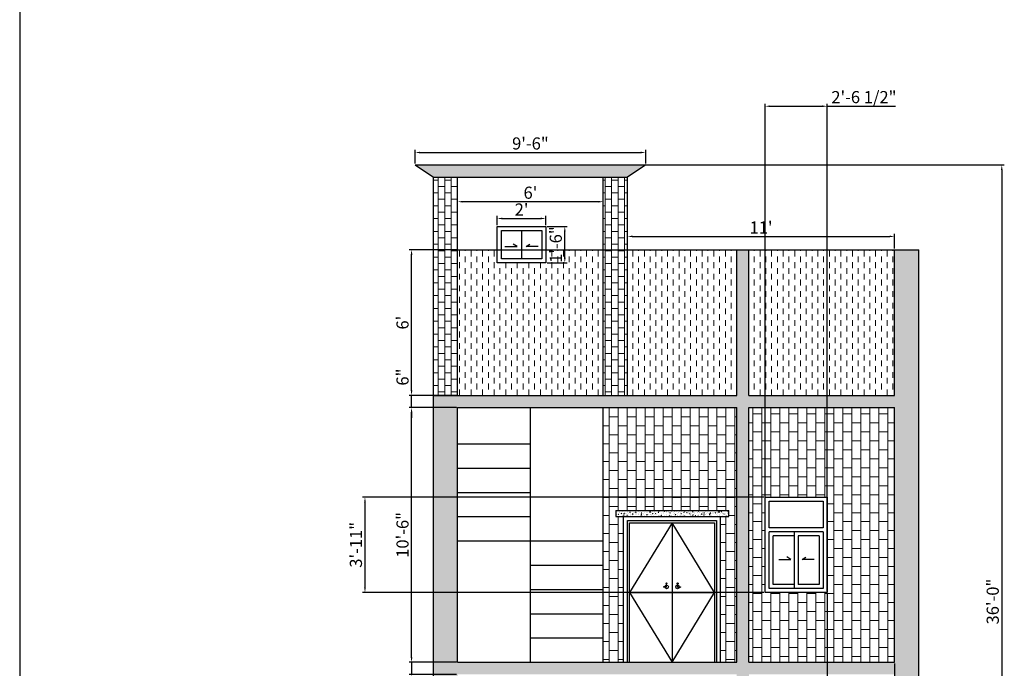
# Model space of a CAD drawing. Units: millimetres. Extents: x 20768 to 23556, y 50760 to 52704.
# Tile 5 of 36: x 20768 to 21255, y 51283 to 51604. Entities that reach past the tile are written whole.
import ezdxf

# ---------------------------------------------------------------- set-up
doc = ezdxf.new("R2010")
doc.units = ezdxf.units.MM
for name, color, linetype, lineweight in [('A-ANNO-DIMS', 2, 'Continuous', 18), ('A-ELEV', 7, 'Continuous', 25), ('A-ELEV-PATT', 8, 'Continuous', 13), ('S-ANNO-DIMS', 2, 'Continuous', 18)]:
    doc.layers.add(name, color=color, linetype=linetype, lineweight=lineweight)
doc.styles.get("Standard").update_dxf_attribs({"font": 'arial.ttf'})
doc.dimstyles.new('ISO-25', dxfattribs={"dimtxt": 6, "dimasz": 2.5, "dimexe": 1.25, "dimexo": 0.625, "dimtad": 1, "dimdec": 0, "dimlunit": 3, "dimtxsty": 'Standard', "dimcen": 2.5, "dimadec": 0, "dimazin": 0, "dimtfac": 1, "dimtdec": 0, "dimtmove": 0, "dimatfit": 3, "dimfxl": 1, "dimarcsym": 0})
pattern_1 = [(90, (105.777, 340.6355), (-3.175, 2e-16), []), (180, (105.777, 340.6355), (-8e-16, -6.35), [3.175, -3.175]), (180, (105.777, 343.8105), (-8e-16, -6.35), [-3.175, 3.175])]
pattern_2 = [(90, (105.777, 340.6355), (-2.8575, 2.8575), [2.8575, -2.8575])]
pattern_3 = [(140, (105.777, 340.6355), (0.23908628, 2.732770035), [0.28575, -3.14325]), (85, (105.777, 340.6355), (-2.86585268, -0.52865132), [0.2286, -2.51460876]), (190.4514447, (105.797, 340.8633), (-2.62676628, 2.20411871), [0.24285013, -2.67135367]), (136.1842, (105.015, 340.6355), (0.63063492, 4.06618561), [0.428625, -4.714875]), (186.635558, (105.0677, 340.9744), (-3.71139187, 3.561062), [0.36427535, -4.00703412]), (81.184151, (105.015, 340.6355), (-3.71139187, 3.561062), [0.3428995, -3.77189598]), (111, (105.2056, 341.0165), (1.53397797, 2.27421587), [0.28575, -3.14325]), (56, (105.2056, 341.0165), (-2.76281949, 0.92703043), [0.2286, -2.5146]), (161.451445, (105.3334, 341.206), (-1.22884153, 3.20124629), [0.24285013, -2.67134906]), (127.5, (105.7771, 340.6355), (-1.268325583, 0.046329049), [0, -2.48412, 0, -2.5527, 0, -2.524125]), (97.5, (105.7771, 340.6355), (-1.502708622, 1.002294938), [0, -1.45542, 0, -2.42697, 0, -0.962025]), (57.5, (105.7771, 339.7859), (0.08593116, 2.033858928), [0, -0.9525, 0, -2.9718, 0, -3.94335]), (47.5, (105.7771, 339.4049), (-0.381397365, 2.22193772), [0, -1.23825, 0, -1.97358, 0, -2.80035])]

# ---------------------------------------------------------------- blocks, each defined once
blk = doc.blocks.new('*D115')
at = {"layer": 'A-ANNO-DIMS', "color": 0, "lineweight": -2, "transparency": 16777216}
for p, q in [((20961.86, 51288.9), (20961.86, 51291.4)), ((20984.01, 51286.4), (20960.61, 51286.4)), ((20961.86, 51286.4), (20961.86, 51280.4)), ((20984.01, 51280.4), (20960.61, 51280.4)), ((20961.86, 51277.9), (20961.86, 51267.22))]:
    blk.add_line(p, q, dxfattribs=at)
at = {"layer": 'A-ANNO-DIMS', "color": 0, "transparency": 16777216}
for points in [[(20961.44, 51288.9), (20962.28, 51288.9), (20961.86, 51286.4)], [(20961.44, 51277.9), (20962.28, 51277.9), (20961.86, 51280.4)]]:
    blk.add_solid(points, dxfattribs=at)
at = {"layer": 'Defpoints', "color": 0, "transparency": 16777216}
for p in [(20984.63, 51286.4), (20961.86, 51280.4), (20984.63, 51280.4)]:
    blk.add_point(p, dxfattribs=at)
at = {"layer": 'A-ANNO-DIMS', "color": 0, "transparency": 16777216, "insert": (20958.17, 51271.31), "char_height": 6, "attachment_point": 5, "rotation": 90}
blk.add_mtext('6"', dxfattribs=at)
blk = doc.blocks.new('*D116')
at = {"layer": 'A-ANNO-DIMS', "color": 0, "lineweight": -2, "transparency": 16777216}
for p, q in [((20984.01, 51412.3), (20960.61, 51412.3)), ((20961.86, 51288.9), (20961.86, 51409.8)), ((20984.01, 51286.4), (20960.61, 51286.4))]:
    blk.add_line(p, q, dxfattribs=at)
at = {"layer": 'A-ANNO-DIMS', "color": 0, "transparency": 16777216}
for points in [[(20961.44, 51409.8), (20962.28, 51409.8), (20961.86, 51412.3)], [(20961.44, 51288.9), (20962.28, 51288.9), (20961.86, 51286.4)]]:
    blk.add_solid(points, dxfattribs=at)
at = {"layer": 'Defpoints', "color": 0, "transparency": 16777216}
for p in [(20961.86, 51412.3), (20984.63, 51412.3), (20984.63, 51286.4)]:
    blk.add_point(p, dxfattribs=at)
at = {"layer": 'A-ANNO-DIMS', "color": 0, "transparency": 16777216, "insert": (20958.17, 51349.35), "char_height": 6, "attachment_point": 5, "rotation": 90}
blk.add_mtext('10\'-6"', dxfattribs=at)
blk = doc.blocks.new('*D117')
at = {"layer": 'A-ANNO-DIMS', "color": 0, "lineweight": -2, "transparency": 16777216}
for p, q in [((20961.86, 51420.8), (20961.86, 51431.48)), ((20984.01, 51418.3), (20960.61, 51418.3)), ((20961.86, 51412.3), (20961.86, 51418.3)), ((20984.01, 51412.3), (20960.61, 51412.3)), ((20961.86, 51409.8), (20961.86, 51407.3))]:
    blk.add_line(p, q, dxfattribs=at)
at = {"layer": 'A-ANNO-DIMS', "color": 0, "transparency": 16777216}
for points in [[(20961.44, 51420.8), (20962.28, 51420.8), (20961.86, 51418.3)], [(20961.44, 51409.8), (20962.28, 51409.8), (20961.86, 51412.3)]]:
    blk.add_solid(points, dxfattribs=at)
at = {"layer": 'Defpoints', "color": 0, "transparency": 16777216}
for p in [(20961.86, 51418.3), (20984.63, 51418.3), (20984.63, 51412.3)]:
    blk.add_point(p, dxfattribs=at)
at = {"layer": 'A-ANNO-DIMS', "color": 0, "transparency": 16777216, "insert": (20958.17, 51427.39), "char_height": 6, "attachment_point": 5, "rotation": 90}
blk.add_mtext('6"', dxfattribs=at)
blk = doc.blocks.new('*D118')
at = {"layer": 'A-ANNO-DIMS', "color": 0, "lineweight": -2, "transparency": 16777216}
for p, q in [((21004.25, 51502.51), (21004.25, 51507.06)), ((21028.25, 51502.51), (21028.25, 51507.06)), ((21006.75, 51505.81), (21025.75, 51505.81))]:
    blk.add_line(p, q, dxfattribs=at)
at = {"layer": 'A-ANNO-DIMS', "color": 0, "transparency": 16777216}
for points in [[(21006.75, 51506.22), (21006.75, 51505.39), (21004.25, 51505.81)], [(21025.75, 51506.22), (21025.75, 51505.39), (21028.25, 51505.81)]]:
    blk.add_solid(points, dxfattribs=at)
at = {"layer": 'Defpoints', "color": 0, "transparency": 16777216}
for p in [(21028.25, 51505.81), (21004.25, 51501.88), (21028.25, 51501.88)]:
    blk.add_point(p, dxfattribs=at)
at = {"layer": 'A-ANNO-DIMS', "color": 0, "transparency": 16777216, "insert": (21016.25, 51509.45), "char_height": 6, "attachment_point": 5}
blk.add_mtext("2'", dxfattribs=at)
blk = doc.blocks.new('*D119')
at = {"layer": 'A-ANNO-DIMS', "color": 0, "lineweight": -2, "transparency": 16777216}
for p, q in [((21028.87, 51501.88), (21038.86, 51501.88)), ((21037.61, 51486.38), (21037.61, 51499.38)), ((21028.87, 51483.88), (21038.86, 51483.88))]:
    blk.add_line(p, q, dxfattribs=at)
at = {"layer": 'A-ANNO-DIMS', "color": 0, "transparency": 16777216}
for points in [[(21037.2, 51499.38), (21038.03, 51499.38), (21037.61, 51501.88)], [(21037.2, 51486.38), (21038.03, 51486.38), (21037.61, 51483.88)]]:
    blk.add_solid(points, dxfattribs=at)
at = {"layer": 'Defpoints', "color": 0, "transparency": 16777216}
for p in [(21028.25, 51501.88), (21037.61, 51501.88), (21028.25, 51483.88)]:
    blk.add_point(p, dxfattribs=at)
at = {"layer": 'A-ANNO-DIMS', "color": 0, "transparency": 16777216, "insert": (21033.93, 51492.88), "char_height": 6, "attachment_point": 5, "rotation": 90}
blk.add_mtext('1\'-6"', dxfattribs=at)
blk = doc.blocks.new('*D120')
at = {"layer": 'A-ANNO-DIMS', "color": 0, "lineweight": -2, "transparency": 16777216}
for p, q in [((20984.01, 51490.3), (20960.61, 51490.3)), ((20961.86, 51420.8), (20961.86, 51487.8)), ((20984.01, 51418.3), (20960.61, 51418.3))]:
    blk.add_line(p, q, dxfattribs=at)
at = {"layer": 'A-ANNO-DIMS', "color": 0, "transparency": 16777216}
for points in [[(20961.44, 51487.8), (20962.28, 51487.8), (20961.86, 51490.3)], [(20961.44, 51420.8), (20962.28, 51420.8), (20961.86, 51418.3)]]:
    blk.add_solid(points, dxfattribs=at)
at = {"layer": 'Defpoints', "color": 0, "transparency": 16777216}
for p in [(20961.86, 51490.3), (20984.63, 51490.3), (20984.63, 51418.3)]:
    blk.add_point(p, dxfattribs=at)
at = {"layer": 'A-ANNO-DIMS', "color": 0, "transparency": 16777216, "insert": (20958.17, 51454.3), "char_height": 6, "attachment_point": 5, "rotation": 90}
blk.add_mtext("6'", dxfattribs=at)
blk = doc.blocks.new('*D121')
at = {"layer": 'A-ANNO-DIMS', "color": 0, "lineweight": -2, "transparency": 16777216}
for p, q in [((20963.6, 51532.92), (20963.6, 51539.67)), ((20966.1, 51538.42), (21075.12, 51538.42)), ((21077.62, 51532.92), (21077.62, 51539.67))]:
    blk.add_line(p, q, dxfattribs=at)
at = {"layer": 'A-ANNO-DIMS', "color": 0, "transparency": 16777216}
for points in [[(20966.1, 51538.83), (20966.1, 51538), (20963.6, 51538.42)], [(21075.12, 51538.83), (21075.12, 51538), (21077.62, 51538.42)]]:
    blk.add_solid(points, dxfattribs=at)
at = {"layer": 'Defpoints', "color": 0, "transparency": 16777216}
for p in [(21077.62, 51538.42), (20963.6, 51532.3), (21077.62, 51532.3)]:
    blk.add_point(p, dxfattribs=at)
at = {"layer": 'A-ANNO-DIMS', "color": 0, "transparency": 16777216, "insert": (21020.61, 51542.11), "char_height": 6, "attachment_point": 5}
blk.add_mtext('9\'-6"', dxfattribs=at)
blk = doc.blocks.new('*D122')
at = {"layer": 'A-ANNO-DIMS', "color": 0, "lineweight": -2, "transparency": 16777216}
for p, q in [((21068.63, 51490.92), (21068.63, 51498.19)), ((21200.63, 51490.92), (21200.63, 51498.19)), ((21071.13, 51496.94), (21198.13, 51496.94))]:
    blk.add_line(p, q, dxfattribs=at)
at = {"layer": 'A-ANNO-DIMS', "color": 0, "transparency": 16777216}
for points in [[(21071.13, 51497.36), (21071.13, 51496.52), (21068.63, 51496.94)], [(21198.13, 51497.36), (21198.13, 51496.52), (21200.63, 51496.94)]]:
    blk.add_solid(points, dxfattribs=at)
at = {"layer": 'Defpoints', "color": 0, "transparency": 16777216}
for p in [(21200.63, 51496.94), (21068.63, 51490.3), (21200.63, 51490.3)]:
    blk.add_point(p, dxfattribs=at)
at = {"layer": 'A-ANNO-DIMS', "color": 0, "transparency": 16777216, "insert": (21134.63, 51500.58), "char_height": 6, "attachment_point": 5}
blk.add_mtext("11'", dxfattribs=at)
blk = doc.blocks.new('*D127')
at = {"layer": 'A-ANNO-DIMS', "color": 0, "lineweight": -2, "transparency": 16777216}
for p, q in [((20984.63, 51490.92), (20984.63, 51515.33)), ((21054.13, 51514.08), (20987.13, 51514.08)), ((21056.63, 51490.92), (21056.63, 51515.33))]:
    blk.add_line(p, q, dxfattribs=at)
at = {"layer": 'A-ANNO-DIMS', "color": 0, "transparency": 16777216}
for points in [[(20987.13, 51514.5), (20987.13, 51513.67), (20984.63, 51514.08)], [(21054.13, 51514.5), (21054.13, 51513.67), (21056.63, 51514.08)]]:
    blk.add_solid(points, dxfattribs=at)
at = {"layer": 'Defpoints', "color": 0, "transparency": 16777216}
for p in [(20984.63, 51514.08), (20984.63, 51490.3), (21056.63, 51490.3)]:
    blk.add_point(p, dxfattribs=at)
at = {"layer": 'A-ANNO-DIMS', "color": 0, "transparency": 16777216, "insert": (21020.63, 51517.77), "char_height": 6, "attachment_point": 5}
blk.add_mtext("6'", dxfattribs=at)
blk = doc.blocks.new('*D129')
at = {"layer": 'A-ANNO-DIMS', "color": 0, "lineweight": -2, "transparency": 16777216}
for p, q in [((21136.01, 51368), (20937.58, 51368)), ((20938.83, 51365.5), (20938.83, 51323.4)), ((21136.01, 51320.9), (20937.58, 51320.9))]:
    blk.add_line(p, q, dxfattribs=at)
at = {"layer": 'A-ANNO-DIMS', "color": 0, "transparency": 16777216}
for points in [[(20938.42, 51365.5), (20939.25, 51365.5), (20938.83, 51368)], [(20938.42, 51323.4), (20939.25, 51323.4), (20938.83, 51320.9)]]:
    blk.add_solid(points, dxfattribs=at)
at = {"layer": 'Defpoints', "color": 0, "transparency": 16777216}
for p in [(21136.63, 51368), (20938.83, 51320.9), (21136.63, 51320.9)]:
    blk.add_point(p, dxfattribs=at)
at = {"layer": 'A-ANNO-DIMS', "color": 0, "transparency": 16777216, "insert": (20935.14, 51344.45), "char_height": 6, "attachment_point": 5, "rotation": 90}
blk.add_mtext('3\'-11"', dxfattribs=at)
blk = doc.blocks.new('*D229')
at = {"layer": 'Defpoints', "color": 0, "transparency": 16777216}
for p in [(20963.6, 51532.3), (20960.63, 51100.5), (21253.63, 51100.5)]:
    blk.add_point(p, dxfattribs=at)
at = {"layer": 'S-ANNO-DIMS', "color": 0, "lineweight": -2, "transparency": 16777216}
for p, q in [((20964.22, 51532.3), (21254.88, 51532.3)), ((21253.63, 51529.8), (21253.63, 51103)), ((20961.26, 51100.5), (21254.88, 51100.5))]:
    blk.add_line(p, q, dxfattribs=at)
at = {"layer": 'S-ANNO-DIMS', "color": 0, "transparency": 16777216}
for points in [[(21253.22, 51529.8), (21254.05, 51529.8), (21253.63, 51532.3)], [(21253.22, 51103), (21254.05, 51103), (21253.63, 51100.5)]]:
    blk.add_solid(points, dxfattribs=at)
at = {"layer": 'S-ANNO-DIMS', "color": 0, "transparency": 16777216, "insert": (21249.94, 51316.4), "char_height": 6, "attachment_point": 5, "rotation": 90}
blk.add_mtext('36\'-0"', dxfattribs=at)
blk = doc.blocks.new('*D230')
at = {"layer": 'Defpoints', "color": 0, "transparency": 16777216}
for p in [(21167.33, 51561.3), (21136.63, 51320.9), (21167.33, 51320.9)]:
    blk.add_point(p, dxfattribs=at)
at = {"layer": 'S-ANNO-DIMS', "color": 0, "lineweight": -2, "transparency": 16777216}
for p, q in [((21136.63, 51321.52), (21136.63, 51562.55)), ((21139.13, 51561.3), (21164.83, 51561.3)), ((21167.33, 51321.52), (21167.33, 51562.55)), ((21167.33, 51561.3), (21201.12, 51561.3))]:
    blk.add_line(p, q, dxfattribs=at)
at = {"layer": 'S-ANNO-DIMS', "color": 0, "transparency": 16777216}
for points in [[(21139.13, 51561.71), (21139.13, 51560.88), (21136.63, 51561.3)], [(21164.83, 51561.71), (21164.83, 51560.88), (21167.33, 51561.3)]]:
    blk.add_solid(points, dxfattribs=at)
at = {"layer": 'S-ANNO-DIMS', "color": 0, "transparency": 16777216, "insert": (21185.48, 51565.03), "char_height": 6, "attachment_point": 5}
blk.add_mtext('2\'-6 1/2"', dxfattribs=at)
blk = doc.blocks.new('*D231')
at = {"layer": 'Defpoints', "color": 0, "transparency": 16777216}
for p in [(21167.33, 51320.9), (21200.63, 51286.4), (21200.63, 51071.5)]:
    blk.add_point(p, dxfattribs=at)
at = {"layer": 'S-ANNO-DIMS', "color": 0, "lineweight": -2, "transparency": 16777216}
for p, q in [((21167.33, 51320.27), (21167.33, 51070.25)), ((21200.63, 51285.77), (21200.63, 51070.25)), ((21169.83, 51071.5), (21198.13, 51071.5))]:
    blk.add_line(p, q, dxfattribs=at)
at = {"layer": 'S-ANNO-DIMS', "color": 0, "transparency": 16777216}
for points in [[(21169.83, 51071.91), (21169.83, 51071.08), (21167.33, 51071.5)], [(21198.13, 51071.91), (21198.13, 51071.08), (21200.63, 51071.5)]]:
    blk.add_solid(points, dxfattribs=at)
at = {"layer": 'S-ANNO-DIMS', "color": 0, "transparency": 16777216, "insert": (21183.98, 51075.23), "char_height": 6, "attachment_point": 5}
blk.add_mtext('2\'-9 1/2"', dxfattribs=at)

msp = doc.modelspace()

# ---------------------------------------------------------------- hatches: boundary and pattern name
at = {"layer": 'A-ELEV-PATT'}
h = msp.add_hatch(dxfattribs=at)
h.set_pattern_fill('AR-CONC', color=256, scale=0.015, angle=90)
h.set_pattern_definition(pattern_3)
h.paths.add_polyline_path([(21077.62, 51532.3), (20963.6, 51532.3), (20972.63, 51526.3), (21068.63, 51526.3)])
h = msp.add_hatch(dxfattribs=at)
h.set_pattern_fill('BRICK', color=256, scale=0.5, angle=90)
h.set_pattern_definition(pattern_1)
h.paths.add_polyline_path([(20984.63, 51526.3), (20972.63, 51526.3), (20972.63, 51418.3), (20984.63, 51418.3)])
h = msp.add_hatch(dxfattribs=at)
h.set_pattern_fill('BRICK', color=256, scale=0.5, angle=90)
h.set_pattern_definition(pattern_1)
h.paths.add_polyline_path([(21068.63, 51526.3), (21056.63, 51526.3), (21056.63, 51490.3), (21068.63, 51490.3)])
h = msp.add_hatch(dxfattribs=at)
h.set_pattern_fill('AR-CONC', color=256, scale=0.015, angle=90)
h.set_pattern_definition(pattern_3)
h.paths.add_polyline_path([(21212.63, 51490.3), (21200.63, 51490.3), (21200.63, 51418.3), (21128.63, 51418.3), (21128.63, 51490.3), (21122.63, 51490.3), (21122.63, 51418.3), (20972.63, 51418.3), (20972.63, 51109.5), (20960.63, 51109.5), (20960.63, 51100.5), (20996.63, 51100.5), (20996.63, 51109.5), (20984.63, 51109.5), (20984.63, 51148.5), (21122.63, 51148.5), (21122.63, 51109.5), (21113.63, 51109.5), (21113.63, 51100.5), (21137.63, 51100.5), (21137.63, 51109.5), (21128.63, 51109.5), (21128.63, 51148.5), (21212.63, 51148.5)])
h.paths.add_polyline_path([(21122.63, 51280.4), (21122.63, 51154.5), (20984.63, 51154.5), (20984.63, 51280.4)], flags=16)
h.paths.add_polyline_path([(21122.63, 51286.4), (20984.63, 51286.4), (20984.63, 51412.3), (21122.63, 51412.3)], flags=16)
h.paths.add_polyline_path([(21128.63, 51280.4), (21200.63, 51280.4), (21200.63, 51154.5), (21128.63, 51154.5)], flags=16)
h.paths.add_polyline_path([(21128.63, 51286.4), (21128.63, 51412.3), (21200.63, 51412.3), (21200.63, 51286.4)], flags=16)
h.paths.add_polyline_path([(21062.79, 51358.4), (21062.79, 51361.4), (21118.63, 51361.4), (21118.63, 51358.4)], flags=0)
h.paths.add_polyline_path([(21111.63, 51320.9), (21090.63, 51286.4), (21069.63, 51320.9), (21069.63, 51355.4), (21111.63, 51355.4)], flags=0)
h.paths.add_polyline_path([(21069.63, 51320.9), (21090.63, 51355.4), (21111.63, 51320.9)], flags=0)
h.paths.add_polyline_path([(21136.63, 51320.9), (21136.63, 51368), (21167.33, 51368), (21167.33, 51320.9)], flags=0)
h.paths.add_polyline_path([(21138.63, 51322.9), (21138.63, 51350.9), (21165.33, 51350.9), (21165.33, 51322.9)], flags=0)
h.paths.add_polyline_path([(21140.63, 51324.9), (21140.63, 51348.9), (21150.98, 51348.9), (21150.98, 51324.9)], flags=0)
h.paths.add_polyline_path([(21136.63, 51236.1), (21167.33, 51236.1), (21167.33, 51189), (21136.63, 51189)], flags=0)
h.paths.add_polyline_path([(21152.98, 51324.9), (21152.98, 51348.9), (21163.33, 51348.9), (21163.33, 51324.9)], flags=0)
h.paths.add_polyline_path([(21094.84, 51323.58), (21094.21, 51323.58, -0.960515), (21092.46, 51323.65, -0.414214), (21093.33, 51324.52), (21093.33, 51325.09, -0.357901), (21093.11, 51325.35, -1), (21093.66, 51325.35, -0.34824), (21093.45, 51325.09), (21093.45, 51324.51, -0.376216), (21094.21, 51323.65), (21094.84, 51323.65)], flags=0)
h.paths.add_polyline_path([(21138.63, 51234.1), (21165.33, 51234.1), (21165.33, 51221), (21138.63, 51221)], flags=0)
h.paths.add_polyline_path([(21118.63, 51229.5), (21118.63, 51226.5), (21062.79, 51226.5), (21062.79, 51229.5)], flags=0)
h.paths.add_polyline_path([(21087.06, 51323.58), (21086.42, 51323.58), (21086.42, 51323.65), (21087.06, 51323.65, -0.376216), (21087.82, 51324.51), (21087.82, 51325.09, -0.34824), (21087.61, 51325.35, -1), (21088.15, 51325.35, -0.357901), (21087.94, 51325.09), (21087.94, 51324.52, -0.414214), (21088.81, 51323.65, -0.960515)], flags=0)
h.paths.add_polyline_path([(21111.63, 51223.5), (21111.63, 51189), (21090.63, 51154.5), (21069.63, 51189), (21069.63, 51223.5)], flags=0)
h.paths.add_polyline_path([(21138.63, 51219), (21165.33, 51219), (21165.33, 51191), (21138.63, 51191)], flags=0)
h.paths.add_polyline_path([(21140.63, 51217), (21150.98, 51217), (21150.98, 51193), (21140.63, 51193)], flags=0)
h.paths.add_polyline_path([(21056.63, 51166.5), (21020.63, 51166.5), (21020.63, 51214.5), (21056.63, 51214.5)], flags=0)
h.paths.add_polyline_path([(21056.63, 51298.4), (21020.63, 51298.4), (21020.63, 51346.4), (21056.63, 51346.4)], flags=0)
h.paths.add_polyline_path([(21090.63, 51223.5), (21111.63, 51189), (21069.63, 51189)], flags=0)
h.paths.add_polyline_path([(21138.63, 51352.9), (21138.63, 51366), (21165.33, 51366), (21165.33, 51352.9)], flags=0)
h.paths.add_polyline_path([(21152.98, 51217), (21163.33, 51217), (21163.33, 51193), (21152.98, 51193)], flags=0)
h.paths.add_polyline_path([(21093.66, 51193.45, -0.34824), (21093.45, 51193.19), (21093.45, 51192.61, -0.376216), (21094.21, 51191.75), (21094.84, 51191.75), (21094.84, 51191.68), (21094.21, 51191.68, -0.960515), (21092.46, 51191.75, -0.414214), (21093.33, 51192.62), (21093.33, 51193.19, -0.357901), (21093.11, 51193.45, -1)], flags=0)
h.paths.add_polyline_path([(21088.15, 51193.45, -0.357901), (21087.94, 51193.19), (21087.94, 51192.62, -0.414214), (21088.81, 51191.75, -0.960515), (21087.06, 51191.68), (21086.42, 51191.68), (21086.42, 51191.75), (21087.06, 51191.75, -0.376216), (21087.82, 51192.61), (21087.82, 51193.19, -0.34824), (21087.61, 51193.45, -1)], flags=0)
h = msp.add_hatch(dxfattribs=at)
h.set_pattern_fill('DASH', color=256, scale=0.9, angle=90)
h.set_pattern_definition(pattern_2)
h.paths.add_polyline_path([(21056.63, 51490.3), (21028.25, 51490.3), (21028.25, 51483.88), (21004.25, 51483.88), (21004.25, 51490.3), (20984.63, 51490.3), (20984.63, 51418.3), (21056.63, 51418.3)])
h = msp.add_hatch(dxfattribs=at)
h.set_pattern_fill('BRICK', color=256, scale=0.5, angle=90)
h.set_pattern_definition(pattern_1)
h.paths.add_polyline_path([(21068.63, 51490.3), (21056.63, 51490.3), (21056.63, 51418.3), (21068.63, 51418.3)])
h = msp.add_hatch(dxfattribs=at)
h.set_pattern_fill('DASH', color=256, scale=0.9, angle=90)
h.set_pattern_definition(pattern_2)
h.paths.add_polyline_path([(21122.63, 51490.3), (21068.63, 51490.3), (21068.63, 51418.3), (21122.63, 51418.3)])
h = msp.add_hatch(dxfattribs=at)
h.set_pattern_fill('DASH', color=256, scale=0.9, angle=90)
h.set_pattern_definition(pattern_2)
h.paths.add_polyline_path([(21200.63, 51490.3), (21128.63, 51490.3), (21128.63, 51418.3), (21200.63, 51418.3)])
h = msp.add_hatch(dxfattribs=at)
h.set_pattern_fill('BRICK', color=256, scale=0.7, angle=90)
h.set_pattern_definition([(90, (105.777, 472.5355), (-4.445, 3e-16), []), (180, (105.777, 472.5355), (-1e-15, -8.89), [4.445, -4.445]), (180, (105.777, 476.9805), (-1e-15, -8.89), [-4.445, 4.445])])
h.paths.add_polyline_path([(21122.63, 51412.3), (21056.63, 51412.3), (21056.63, 51286.4), (21066.63, 51286.4), (21066.63, 51358.4), (21062.79, 51358.4), (21062.79, 51361.4), (21118.63, 51361.4), (21118.63, 51358.4), (21114.63, 51358.4), (21114.63, 51286.4), (21122.63, 51286.4)])
h = msp.add_hatch(dxfattribs=at)
h.set_pattern_fill('BRICK', color=256, scale=0.7, angle=90)
h.set_pattern_definition([(90, (105.777, 340.6355), (-4.445, 3e-16), []), (180, (105.777, 340.6355), (-1e-15, -8.89), [4.445, -4.445]), (180, (105.777, 345.0805), (-1e-15, -8.89), [-4.445, 4.445])])
h.paths.add_polyline_path([(21200.63, 51412.3), (21128.63, 51412.3), (21128.63, 51286.4), (21200.63, 51286.4)])
h.paths.add_polyline_path([(21167.33, 51320.9), (21136.63, 51320.9), (21136.63, 51368), (21167.33, 51368)], flags=16)
h.paths.add_polyline_path([(21165.33, 51350.9), (21165.33, 51322.9), (21138.63, 51322.9), (21138.63, 51350.9)], flags=0)
h.paths.add_polyline_path([(21165.33, 51352.9), (21138.63, 51352.9), (21138.63, 51366), (21165.33, 51366)], flags=0)
h.paths.add_polyline_path([(21163.33, 51348.9), (21163.33, 51324.9), (21152.98, 51324.9), (21152.98, 51348.9)], flags=0)
h.paths.add_polyline_path([(21150.98, 51324.9), (21140.63, 51324.9), (21140.63, 51348.9), (21150.98, 51348.9)], flags=0)
h = msp.add_hatch(dxfattribs=at)
h.set_pattern_fill('AR-CONC', color=256, scale=0.015, angle=90)
h.paths.add_polyline_path([(21118.63, 51361.4), (21062.79, 51361.4), (21062.79, 51358.4), (21118.63, 51358.4)])

# ---------------------------------------------------------------- linework, layer by layer
at = {"layer": 'A-ELEV'}
for p, q in [((20768.14, 51623.53), (20768.14, 50975.78)), ((20963.6, 51532.3), (21077.62, 51532.3)), ((20963.6, 51532.3), (20972.63, 51526.3)), ((21077.62, 51532.3), (21068.63, 51526.3)), ((20972.63, 51109.5), (20972.63, 51526.3)), ((20972.63, 51526.3), (21068.63, 51526.3)), ((20984.63, 51418.3), (20984.63, 51526.3)), ((21056.63, 51418.3), (21056.63, 51526.3)), ((21068.63, 51418.3), (21068.63, 51526.3)), ((21016.25, 51499.88), (21016.25, 51485.88)), ((21014, 51491.87), (21012.1, 51493.08)), ((21018.5, 51491.87), (21020.39, 51493.08)), ((20984.63, 51490.3), (21212.63, 51490.3)), ((21008.02, 51491.87), (21014, 51491.87)), ((21024.48, 51491.87), (21018.5, 51491.87)), ((21122.63, 51418.3), (21122.63, 51490.3)), ((21128.63, 51418.3), (21128.63, 51490.3)), ((21200.63, 51418.3), (21200.63, 51490.3)), ((21212.63, 51109.5), (21212.63, 51490.3)), ((20972.63, 51418.3), (21122.63, 51418.3)), ((21128.63, 51418.3), (21200.63, 51418.3)), ((20984.63, 51286.4), (20984.63, 51412.3)), ((20984.63, 51412.3), (21122.63, 51412.3)), ((21020.63, 51286.4), (21020.63, 51412.3)), ((21056.63, 51286.4), (21056.63, 51412.3)), ((21122.63, 51286.4), (21122.63, 51412.3)), ((21128.63, 51286.4), (21128.63, 51412.3)), ((21128.63, 51412.3), (21200.63, 51412.3)), ((21200.63, 51286.4), (21200.63, 51412.3)), ((20984.63, 51394.4), (21020.63, 51394.4)), ((20984.63, 51382.4), (21020.63, 51382.4)), ((20984.63, 51370.4), (21020.63, 51370.4)), ((21136.63, 51368), (21167.33, 51368)), ((21136.63, 51320.9), (21136.63, 51368)), ((21167.33, 51368), (21167.33, 51320.9)), ((21062.79, 51361.4), (21118.63, 51361.4)), ((21062.79, 51361.4), (21062.79, 51358.4)), ((21118.63, 51358.4), (21118.63, 51361.4)), ((20984.63, 51358.4), (21020.63, 51358.4)), ((21062.79, 51358.4), (21118.63, 51358.4)), ((21066.63, 51286.4), (21066.63, 51358.4)), ((21114.63, 51286.4), (21114.63, 51358.4)), ((21090.63, 51355.4), (21069.63, 51320.9)), ((21090.63, 51355.4), (21090.63, 51286.4)), ((21111.63, 51320.9), (21090.63, 51355.4)), ((20984.63, 51346.4), (21056.63, 51346.4)), ((21165.33, 51350.9), (21138.63, 51350.9)), ((21138.63, 51322.9), (21138.63, 51350.9)), ((21150.98, 51348.9), (21140.63, 51348.9)), ((21140.63, 51324.9), (21140.63, 51348.9)), ((21150.98, 51350.9), (21150.98, 51322.9)), ((21163.33, 51348.9), (21152.98, 51348.9)), ((21152.98, 51348.9), (21152.98, 51324.9)), ((21163.33, 51348.9), (21163.33, 51324.9)), ((21165.33, 51350.9), (21165.33, 51322.9)), ((21143.34, 51337.27), (21149.32, 51337.27)), ((21149.32, 51337.27), (21147.43, 51338.48)), ((21154.92, 51337.2), (21156.81, 51338.41)), ((21160.9, 51337.2), (21154.92, 51337.2)), ((21020.63, 51334.4), (21056.63, 51334.4)), ((21020.63, 51322.4), (21056.63, 51322.4)), ((21087.82, 51323.65), (21086.42, 51323.65)), ((21086.42, 51323.65), (21086.42, 51323.58)), ((21087.94, 51323.58), (21086.42, 51323.58)), ((21087.82, 51323.65), (21087.82, 51325.09)), ((21087.94, 51323.58), (21087.94, 51325.09)), ((21093.33, 51323.58), (21093.33, 51325.09)), ((21093.33, 51323.58), (21094.84, 51323.58)), ((21093.45, 51323.65), (21093.45, 51325.09)), ((21093.45, 51323.65), (21094.84, 51323.65)), ((21094.84, 51323.65), (21094.84, 51323.58)), ((21165.33, 51322.9), (21138.63, 51322.9)), ((21150.98, 51324.9), (21140.63, 51324.9)), ((21163.33, 51324.9), (21152.98, 51324.9)), ((21069.63, 51320.9), (21090.63, 51286.4)), ((21069.63, 51320.9), (21111.63, 51320.9)), ((21090.63, 51286.4), (21111.63, 51320.9)), ((21167.33, 51320.9), (21136.63, 51320.9)), ((21020.63, 51310.4), (21056.63, 51310.4)), ((21020.63, 51298.4), (21056.63, 51298.4)), ((20984.63, 51286.4), (21122.63, 51286.4)), ((21128.63, 51286.4), (21200.63, 51286.4))]:
    msp.add_line(p, q, dxfattribs=at)
for points in [[(21004.25, 51501.88), (21028.25, 51501.88), (21028.25, 51483.88), (21004.25, 51483.88)], [(21006.25, 51499.88), (21026.25, 51499.88), (21026.25, 51485.88), (21006.25, 51485.88)], [(21165.33, 51366), (21165.33, 51352.9), (21138.63, 51352.9), (21138.63, 51366)]]:
    msp.add_lwpolyline(points, close=True, dxfattribs=at)
for points in [[(21068.63, 51286.4), (21068.63, 51356.4), (21112.63, 51356.4), (21112.63, 51286.4)], [(21069.63, 51286.4), (21069.63, 51355.4), (21111.63, 51355.4), (21111.63, 51286.4)]]:
    msp.add_lwpolyline(points, dxfattribs=at)
for centre, radius in [((21087.94, 51323.65), 0.877), ((21087.88, 51325.35), 0.272), ((21093.33, 51323.65), 0.877), ((21093.39, 51325.35), 0.272)]:
    msp.add_circle(centre, radius, dxfattribs=at)

# ---------------------------------------------------------------- dimensions: what is measured, and where the dimension line sits
at = {"layer": 'A-ANNO-DIMS'}
for base, p1, p2, picture, middle in [((21077.62, 51538.42), (20963.6, 51532.3), (21077.62, 51532.3), '*D121', (21020.61, 51542.11)), ((20984.63, 51514.08), (21056.63, 51490.3), (20984.63, 51490.3), '*D127', (21020.63, 51517.77)), ((21028.25, 51505.81), (21004.25, 51501.88), (21028.25, 51501.88), '*D118', (21016.25, 51509.45)), ((21200.63, 51496.94), (21068.63, 51490.3), (21200.63, 51490.3), '*D122', (21134.63, 51500.58))]:
    dim = msp.add_linear_dim(base=base, p1=p1, p2=p2, dimstyle='ISO-25', override={"dimclrd": 0, "dimclre": 0, "dimclrt": 0}, dxfattribs=at)
    dim.commit()
    dim.dimension.update_dxf_attribs({"geometry": picture, "text_midpoint": middle})
for base, p1, p2, picture, middle in [((21037.61, 51501.88), (21028.25, 51483.88), (21028.25, 51501.88), '*D119', (21033.93, 51492.88)), ((20961.86, 51490.3), (20984.63, 51418.3), (20984.63, 51490.3), '*D120', (20958.17, 51454.3)), ((20961.86, 51418.3), (20984.63, 51412.3), (20984.63, 51418.3), '*D117', (20958.17, 51427.39)), ((20961.86, 51412.3), (20984.63, 51286.4), (20984.63, 51412.3), '*D116', (20958.17, 51349.35)), ((20938.83, 51320.9), (21136.63, 51368), (21136.63, 51320.9), '*D129', (20935.14, 51344.45)), ((20961.86, 51280.4), (20984.63, 51286.4), (20984.63, 51280.4), '*D115', (20958.17, 51271.31))]:
    dim = msp.add_linear_dim(base=base, p1=p1, p2=p2, angle=90, dimstyle='ISO-25', override={"dimclrd": 0, "dimclre": 0, "dimclrt": 0}, dxfattribs=at)
    dim.commit()
    dim.dimension.update_dxf_attribs({"geometry": picture, "text_midpoint": middle})
at = {"layer": 'S-ANNO-DIMS'}
for base, p1, p2, picture, middle in [((21167.33, 51561.3), (21136.63, 51320.9), (21167.33, 51320.9), '*D230', (21185.48, 51565.03)), ((21200.63, 51071.5), (21167.33, 51320.9), (21200.63, 51286.4), '*D231', (21183.98, 51075.23))]:
    dim = msp.add_linear_dim(base=base, p1=p1, p2=p2, dimstyle='ISO-25', override={"dimdec": 1, "dimlfac": 1, "dimrnd": 0, "dimzin": 1, "dimdsep": 46, "dimlunit": 4, "dimfrac": 2}, dxfattribs=at)
    dim.commit()
    dim.dimension.update_dxf_attribs({"geometry": picture, "text_midpoint": middle})
dim = msp.add_linear_dim(base=(21253.63, 51100.5), p1=(20963.6, 51532.3), p2=(20960.63, 51100.5), angle=90, dimstyle='ISO-25', override={"dimdec": 1, "dimlfac": 1, "dimrnd": 0, "dimzin": 1, "dimdsep": 46, "dimlunit": 4, "dimfrac": 2}, dxfattribs=at)
dim.commit()
dim.dimension.update_dxf_attribs({"geometry": '*D229', "text_midpoint": (21249.94, 51316.4)})

doc.saveas('drawing.dxf')
